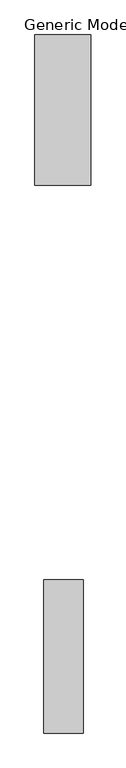
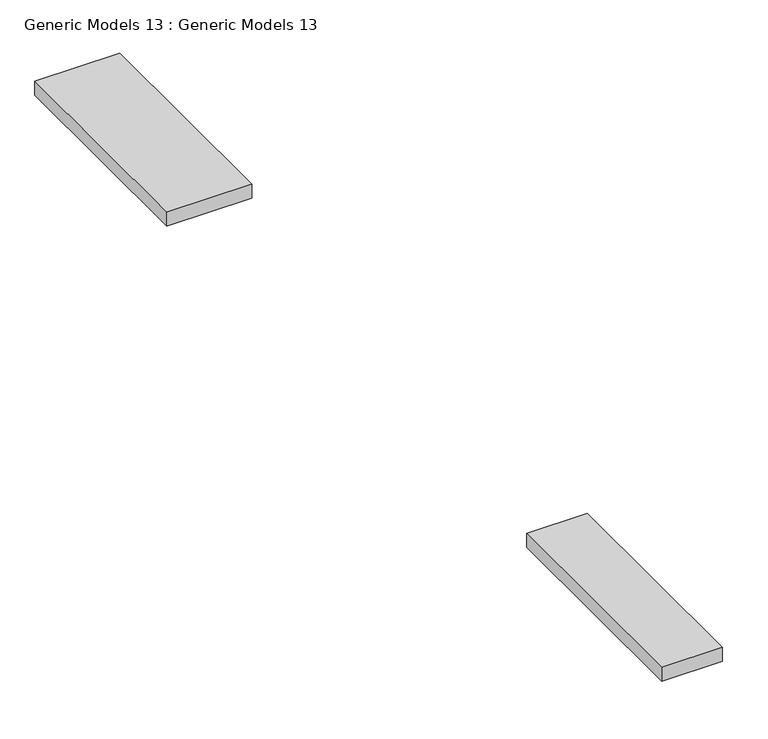
"""IFC4 building model written with IfcOpenShell, lengths in millimetres: proxy geometry, Generic Models 13 : Generic Models 13."""

from ifc_helpers import new_model, si_unit, frame, origin, place, context, project, spatial, polyline, outline, extrude, source, transform, mapped, element, save


def generic_models_13_generic_models_13_81a3a1d9(model_context):
    return source(origin(), model_context, "Body", "SweptSolid", [
        extrude(outline(polyline([(-16847.8054227, -8207.5302573), (-16223.0859258, -8207.5302573), (-16223.0859258, -10619.9777232), (-16847.8054227, -10619.9777232), (-16847.8054227, -8207.5302573)])), frame((0.0, 0.0, 5598.9809912), z_axis=(0.0, 0.0, 1.0), x_axis=(1.0, 0.0, 0.0)), (0.0, 0.0, 1.0), 152.4),
        extrude(outline(polyline([(-16985.0859258, 353.6460165), (-16108.7859258, 353.6460165), (-16108.7859258, -2009.3777232), (-16985.0859258, -2009.3777232), (-16985.0859258, 353.6460165)])), frame((0.0, 0.0, 5399.696684), z_axis=(0.0, 0.0, 1.0), x_axis=(1.0, 0.0, 0.0)), (0.0, 0.0, 1.0), 152.4),
    ])


if __name__ == "__main__":
    model = new_model("IFC4")
    model_context = context("Model", 3, world=origin())
    ifc_project = project(units=[si_unit("LENGTHUNIT", "METRE", prefix="MILLI")], contexts=[model_context])
    site = spatial("IfcSite", under=ifc_project)
    building = spatial("IfcBuilding", under=site)
    placement = place(None, origin())
    generic_models_13_generic_models_13_shape = generic_models_13_generic_models_13_81a3a1d9(model_context)
    element("IfcBuildingElementProxy", 1, Name="Generic Models 13 : Generic Models 13", ObjectType="Generic Models 13 : Generic Models 13", at=placement, inside=building, context=model_context, shape_type="MappedRepresentation", body=[
        mapped(generic_models_13_generic_models_13_shape, transform((0.0, 0.0, 0.0), x_axis=(1.0, 0.0, 0.0), y_axis=(0.0, 1.0, 0.0), z_axis=(0.0, 0.0, 1.0))),
    ])
    save(model, "model.ifc")
